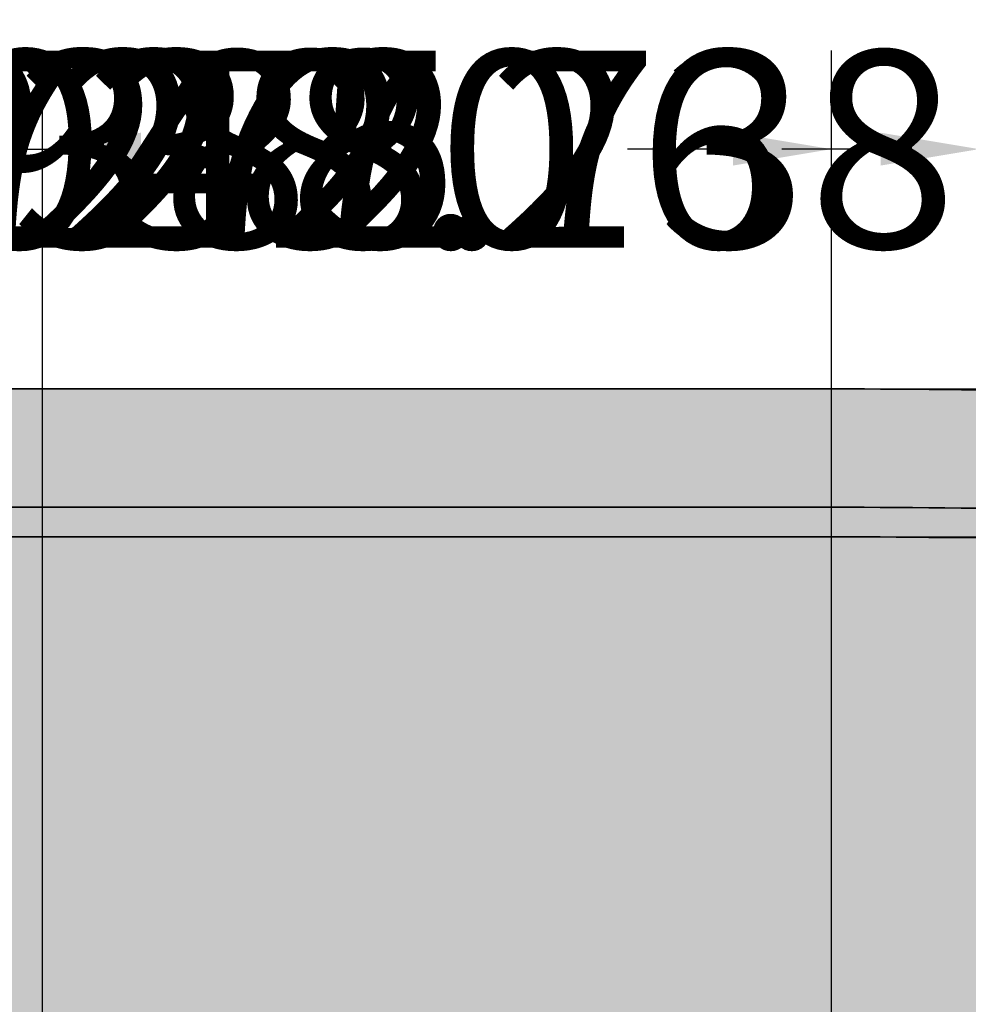
# Model space of a CAD drawing. Units: millimetres. Extents: x 130 to 1021, y 147 to 699.
# Tile 38 of 40: x 550 to 646, y 600 to 699. Entities that reach past the tile are written whole.
import ezdxf

# ---------------------------------------------------------------- set-up
doc = ezdxf.new("R2010")
doc.units = ezdxf.units.MM
doc.header["$MEASUREMENT"] = 0
for name, color, linetype, lineweight in [('A-ANNO-DIMS', 2, 'Continuous', 18), ('A-ELEV', 7, 'Continuous', 35), ('A-ELEV-PATT', 9, 'Continuous', 13)]:
    doc.layers.add(name, color=color, linetype=linetype, lineweight=lineweight)
doc.styles.get("Standard").update_dxf_attribs({"font": 'arial.ttf'})
doc.dimstyles.get("Standard").update_dxf_attribs({"dimtxt": 20, "dimasz": 10, "dimexe": 10, "dimexo": 10, "dimgap": 5, "dimtad": 0, "dimtih": 1, "dimtoh": 1, "dimdec": 0, "dimzin": 0, "dimdsep": 46, "dimtxsty": 'Standard', "dimcen": 5, "dimadec": 0, "dimazin": 0, "dimtfac": 1, "dimtdec": 0, "dimtofl": 0, "dimtmove": 0, "dimatfit": 3, "dimfxl": 1, "dimtolj": 1, "dimtzin": 0, "dimarcsym": 0})

# ---------------------------------------------------------------- blocks, each defined once
blk = doc.blocks.new('*D11')
at = {"layer": 'A-ANNO-DIMS', "color": 0, "lineweight": -2, "transparency": 16777216}
for p, q in [((737.374, 648.699), (737.374, 149.739)), ((299.374, 566.947), (299.374, 149.739)), ((309.374, 159.739), (490.857, 159.739)), ((727.374, 159.739), (545.891, 159.739))]:
    blk.add_line(p, q, dxfattribs=at)
at = {"layer": 'A-ANNO-DIMS', "color": 0, "transparency": 16777216}
for points in [[(309.374, 161.406), (309.374, 158.073), (299.374, 159.739)], [(727.374, 161.406), (727.374, 158.073), (737.374, 159.739)]]:
    blk.add_solid(points, dxfattribs=at)
at = {"layer": 'Defpoints', "color": 0, "transparency": 16777216}
for p in [(737.374, 658.699), (299.374, 576.947), (737.374, 159.739)]:
    blk.add_point(p, dxfattribs=at)
at = {"layer": 'A-ANNO-DIMS', "color": 0, "transparency": 16777216, "insert": (518.374, 159.739), "char_height": 20, "attachment_point": 5}
blk.add_mtext('\\A1;438', dxfattribs=at)
blk = doc.blocks.new('*D22')
at = {"layer": 'A-ANNO-DIMS', "color": 0, "lineweight": -2, "transparency": 16777216}
for p, q in [((447.374, 656.947), (447.374, 696.247)), ((466.767, 403.947), (466.767, 696.247)), ((437.374, 686.247), (427.374, 686.247)), ((476.767, 686.247), (486.767, 686.247))]:
    blk.add_line(p, q, dxfattribs=at)
at = {"layer": 'A-ANNO-DIMS', "color": 0, "transparency": 16777216}
for points in [[(437.374, 687.914), (437.374, 684.581), (447.374, 686.247)], [(476.767, 687.914), (476.767, 684.581), (466.767, 686.247)]]:
    blk.add_solid(points, dxfattribs=at)
at = {"layer": 'Defpoints', "color": 0, "transparency": 16777216}
for p in [(466.767, 686.247), (447.374, 646.947), (466.767, 393.947)]:
    blk.add_point(p, dxfattribs=at)
at = {"layer": 'A-ANNO-DIMS', "color": 0, "transparency": 16777216, "insert": (532.34, 686.247), "char_height": 20, "attachment_point": 5}
blk.add_mtext('\\A1;19.393', dxfattribs=at)
blk = doc.blocks.new('*D23')
at = {"layer": 'A-ANNO-DIMS', "color": 0, "lineweight": -2, "transparency": 16777216}
for p, q in [((466.767, 403.947), (466.767, 696.247)), ((475.988, 209.039), (475.988, 696.247)), ((456.767, 686.247), (446.767, 686.247)), ((485.988, 686.247), (495.988, 686.247))]:
    blk.add_line(p, q, dxfattribs=at)
at = {"layer": 'A-ANNO-DIMS', "color": 0, "transparency": 16777216}
for points in [[(456.767, 687.914), (456.767, 684.581), (466.767, 686.247)], [(485.988, 687.914), (485.988, 684.581), (475.988, 686.247)]]:
    blk.add_solid(points, dxfattribs=at)
at = {"layer": 'Defpoints', "color": 0, "transparency": 16777216}
for p in [(475.988, 686.247), (466.767, 393.947), (475.988, 199.039)]:
    blk.add_point(p, dxfattribs=at)
at = {"layer": 'A-ANNO-DIMS', "color": 0, "transparency": 16777216, "insert": (534.631, 686.247), "char_height": 20, "attachment_point": 5}
blk.add_mtext('\\A1;9.222', dxfattribs=at)
blk = doc.blocks.new('*D24')
at = {"layer": 'A-ANNO-DIMS', "color": 0, "lineweight": -2, "transparency": 16777216}
for p, q in [((475.988, 209.039), (475.988, 696.247)), ((487.374, 671.947), (487.374, 696.247)), ((465.988, 686.247), (455.988, 686.247)), ((497.374, 686.247), (507.374, 686.247))]:
    blk.add_line(p, q, dxfattribs=at)
at = {"layer": 'A-ANNO-DIMS', "color": 0, "transparency": 16777216}
for points in [[(465.988, 687.914), (465.988, 684.581), (475.988, 686.247)], [(497.374, 687.914), (497.374, 684.581), (487.374, 686.247)]]:
    blk.add_solid(points, dxfattribs=at)
at = {"layer": 'Defpoints', "color": 0, "transparency": 16777216}
for p in [(487.374, 686.247), (487.374, 661.947), (475.988, 199.039)]:
    blk.add_point(p, dxfattribs=at)
at = {"layer": 'A-ANNO-DIMS', "color": 0, "transparency": 16777216, "insert": (553.022, 686.247), "char_height": 20, "attachment_point": 5}
blk.add_mtext('\\A1;11.385', dxfattribs=at)
blk = doc.blocks.new('*D25')
at = {"layer": 'A-ANNO-DIMS', "color": 0, "lineweight": -2, "transparency": 16777216}
for p, q in [((487.374, 671.947), (487.374, 696.247)), ((494.102, 506.908), (494.102, 696.247)), ((477.374, 686.247), (467.374, 686.247)), ((504.102, 686.247), (514.102, 686.247))]:
    blk.add_line(p, q, dxfattribs=at)
at = {"layer": 'A-ANNO-DIMS', "color": 0, "transparency": 16777216}
for points in [[(477.374, 687.914), (477.374, 684.581), (487.374, 686.247)], [(504.102, 687.914), (504.102, 684.581), (494.102, 686.247)]]:
    blk.add_solid(points, dxfattribs=at)
at = {"layer": 'Defpoints', "color": 0, "transparency": 16777216}
for p in [(494.102, 686.247), (487.374, 661.947), (494.102, 496.908)]:
    blk.add_point(p, dxfattribs=at)
at = {"layer": 'A-ANNO-DIMS', "color": 0, "transparency": 16777216, "insert": (552.922, 686.247), "char_height": 20, "attachment_point": 5}
blk.add_mtext('\\A1;6.728', dxfattribs=at)
blk = doc.blocks.new('*D26')
at = {"layer": 'A-ANNO-DIMS', "color": 0, "lineweight": -2, "transparency": 16777216}
for p, q in [((494.102, 506.908), (494.102, 696.247)), ((502.374, 593.947), (502.374, 696.247)), ((484.102, 686.247), (474.102, 686.247)), ((512.374, 686.247), (522.374, 686.247))]:
    blk.add_line(p, q, dxfattribs=at)
at = {"layer": 'A-ANNO-DIMS', "color": 0, "transparency": 16777216}
for points in [[(484.102, 687.914), (484.102, 684.581), (494.102, 686.247)], [(512.374, 687.914), (512.374, 684.581), (502.374, 686.247)]]:
    blk.add_solid(points, dxfattribs=at)
at = {"layer": 'Defpoints', "color": 0, "transparency": 16777216}
for p in [(502.374, 686.247), (502.374, 583.947), (494.102, 496.908)]:
    blk.add_point(p, dxfattribs=at)
at = {"layer": 'A-ANNO-DIMS', "color": 0, "transparency": 16777216, "insert": (561.03, 686.247), "char_height": 20, "attachment_point": 5}
blk.add_mtext('\\A1;8.272', dxfattribs=at)
blk = doc.blocks.new('*D27')
at = {"layer": 'A-ANNO-DIMS', "color": 0, "lineweight": -2, "transparency": 16777216}
for p, q in [((502.374, 593.947), (502.374, 696.247)), ((544.635, 396.264), (544.635, 696.247)), ((512.374, 686.247), (534.635, 686.247)), ((544.635, 686.247), (554.635, 686.247))]:
    blk.add_line(p, q, dxfattribs=at)
at = {"layer": 'A-ANNO-DIMS', "color": 0, "transparency": 16777216}
for points in [[(512.374, 687.914), (512.374, 684.581), (502.374, 686.247)], [(534.635, 687.914), (534.635, 684.581), (544.635, 686.247)]]:
    blk.add_solid(points, dxfattribs=at)
at = {"layer": 'Defpoints', "color": 0, "transparency": 16777216}
for p in [(544.635, 686.247), (502.374, 583.947), (544.635, 386.264)]:
    blk.add_point(p, dxfattribs=at)
at = {"layer": 'A-ANNO-DIMS', "color": 0, "transparency": 16777216, "insert": (593.776, 686.247), "char_height": 20, "attachment_point": 5}
blk.add_mtext('\\A1;42.26', dxfattribs=at)
blk = doc.blocks.new('*D28')
at = {"layer": 'A-ANNO-DIMS', "color": 0, "lineweight": -2, "transparency": 16777216}
for p, q in [((544.635, 396.264), (544.635, 696.247)), ((552.374, 593.947), (552.374, 696.247)), ((534.635, 686.247), (524.635, 686.247)), ((562.374, 686.247), (572.374, 686.247))]:
    blk.add_line(p, q, dxfattribs=at)
at = {"layer": 'A-ANNO-DIMS', "color": 0, "transparency": 16777216}
for points in [[(534.635, 687.914), (534.635, 684.581), (544.635, 686.247)], [(562.374, 687.914), (562.374, 684.581), (552.374, 686.247)]]:
    blk.add_solid(points, dxfattribs=at)
at = {"layer": 'Defpoints', "color": 0, "transparency": 16777216}
for p in [(552.374, 686.247), (552.374, 583.947), (544.635, 386.264)]:
    blk.add_point(p, dxfattribs=at)
at = {"layer": 'A-ANNO-DIMS', "color": 0, "transparency": 16777216, "insert": (611.057, 686.247), "char_height": 20, "attachment_point": 5}
blk.add_mtext('\\A1;7.738', dxfattribs=at)
blk = doc.blocks.new('*D29')
at = {"layer": 'A-ANNO-DIMS', "color": 0, "lineweight": -2, "transparency": 16777216}
for p, q in [((552.374, 593.947), (552.374, 696.247)), ((632.374, 593.947), (632.374, 696.247)), ((562.374, 686.247), (573.07, 686.247)), ((622.374, 686.247), (611.678, 686.247))]:
    blk.add_line(p, q, dxfattribs=at)
at = {"layer": 'A-ANNO-DIMS', "color": 0, "transparency": 16777216}
for points in [[(562.374, 687.914), (562.374, 684.581), (552.374, 686.247)], [(622.374, 687.914), (622.374, 684.581), (632.374, 686.247)]]:
    blk.add_solid(points, dxfattribs=at)
at = {"layer": 'Defpoints', "color": 0, "transparency": 16777216}
for p in [(632.374, 686.247), (552.374, 583.947), (632.374, 583.947)]:
    blk.add_point(p, dxfattribs=at)
at = {"layer": 'A-ANNO-DIMS', "color": 0, "transparency": 16777216, "insert": (592.374, 686.247), "char_height": 20, "attachment_point": 5}
blk.add_mtext('\\A1;80', dxfattribs=at)
blk = doc.blocks.new('*D30')
at = {"layer": 'A-ANNO-DIMS', "color": 0, "lineweight": -2, "transparency": 16777216}
for p, q in [((632.374, 593.947), (632.374, 696.247)), ((647.339, 584.979), (647.339, 696.247)), ((622.374, 686.247), (612.374, 686.247)), ((657.339, 686.247), (667.339, 686.247))]:
    blk.add_line(p, q, dxfattribs=at)
at = {"layer": 'A-ANNO-DIMS', "color": 0, "transparency": 16777216}
for points in [[(622.374, 687.914), (622.374, 684.581), (632.374, 686.247)], [(657.339, 687.914), (657.339, 684.581), (647.339, 686.247)]]:
    blk.add_solid(points, dxfattribs=at)
at = {"layer": 'Defpoints', "color": 0, "transparency": 16777216}
for p in [(647.339, 686.247), (632.374, 583.947), (647.339, 574.979)]:
    blk.add_point(p, dxfattribs=at)
at = {"layer": 'A-ANNO-DIMS', "color": 0, "transparency": 16777216, "insert": (712.987, 686.247), "char_height": 20, "attachment_point": 5}
blk.add_mtext('\\A1;14.965', dxfattribs=at)
blk = doc.blocks.new('*D31')
at = {"layer": 'A-ANNO-DIMS', "color": 0, "lineweight": -2, "transparency": 16777216}
for p, q in [((647.339, 584.979), (647.339, 696.247)), ((732.374, 653.96), (732.374, 696.247)), ((637.339, 686.247), (627.339, 686.247)), ((742.374, 686.247), (752.374, 686.247))]:
    blk.add_line(p, q, dxfattribs=at)
at = {"layer": 'A-ANNO-DIMS', "color": 0, "transparency": 16777216}
for points in [[(637.339, 687.914), (637.339, 684.581), (647.339, 686.247)], [(742.374, 687.914), (742.374, 684.581), (732.374, 686.247)]]:
    blk.add_solid(points, dxfattribs=at)
at = {"layer": 'Defpoints', "color": 0, "transparency": 16777216}
for p in [(732.374, 686.247), (732.374, 643.96), (647.339, 574.979)]:
    blk.add_point(p, dxfattribs=at)
at = {"layer": 'A-ANNO-DIMS', "color": 0, "transparency": 16777216, "insert": (689.857, 686.247), "char_height": 20, "attachment_point": 5}
blk.add_mtext('\\A1;85.03', dxfattribs=at)
blk = doc.blocks.new('*D57')
at = {"layer": 'A-ANNO-DIMS', "color": 0, "lineweight": -2, "transparency": 16777216}
for p, q in [((761.674, 606.947), (761.674, 616.947)), ((761.674, 616.947), (771.674, 616.947)), ((497.374, 596.947), (771.674, 596.947)), ((562.374, 583.947), (771.674, 583.947)), ((761.674, 573.947), (761.674, 563.947))]:
    blk.add_line(p, q, dxfattribs=at)
at = {"layer": 'A-ANNO-DIMS', "color": 0, "transparency": 16777216}
for points in [[(760.007, 606.947), (763.34, 606.947), (761.674, 596.947)], [(760.007, 573.947), (763.34, 573.947), (761.674, 583.947)]]:
    blk.add_solid(points, dxfattribs=at)
at = {"layer": 'Defpoints', "color": 0, "transparency": 16777216}
for p in [(487.374, 596.947), (761.674, 596.947), (552.374, 583.947)]:
    blk.add_point(p, dxfattribs=at)
at = {"layer": 'A-ANNO-DIMS', "color": 0, "transparency": 16777216, "insert": (790.057, 616.947), "char_height": 20, "attachment_point": 5}
blk.add_mtext('\\A1;13', dxfattribs=at)
blk = doc.blocks.new('*D58')
at = {"layer": 'A-ANNO-DIMS', "color": 0, "lineweight": -2, "transparency": 16777216}
for p, q in [((761.674, 656.947), (761.674, 666.947)), ((497.374, 646.947), (771.674, 646.947)), ((497.374, 596.947), (771.674, 596.947)), ((761.674, 586.947), (761.674, 576.947))]:
    blk.add_line(p, q, dxfattribs=at)
at = {"layer": 'A-ANNO-DIMS', "color": 0, "transparency": 16777216}
for points in [[(760.007, 656.947), (763.34, 656.947), (761.674, 646.947)], [(760.007, 586.947), (763.34, 586.947), (761.674, 596.947)]]:
    blk.add_solid(points, dxfattribs=at)
at = {"layer": 'Defpoints', "color": 0, "transparency": 16777216}
for p in [(487.374, 646.947), (761.674, 646.947), (487.374, 596.947)]:
    blk.add_point(p, dxfattribs=at)
at = {"layer": 'A-ANNO-DIMS', "color": 0, "transparency": 16777216, "insert": (761.674, 621.947), "char_height": 20, "attachment_point": 5}
blk.add_mtext('\\A1;50', dxfattribs=at)
blk = doc.blocks.new('*D59')
at = {"layer": 'A-ANNO-DIMS', "color": 0, "lineweight": -2, "transparency": 16777216}
for p, q in [((761.674, 671.947), (761.674, 681.947)), ((761.674, 681.947), (771.674, 681.947)), ((497.374, 661.947), (771.674, 661.947)), ((497.374, 646.947), (771.674, 646.947)), ((761.674, 636.947), (761.674, 626.947))]:
    blk.add_line(p, q, dxfattribs=at)
at = {"layer": 'A-ANNO-DIMS', "color": 0, "transparency": 16777216}
for points in [[(760.007, 671.947), (763.34, 671.947), (761.674, 661.947)], [(760.007, 636.947), (763.34, 636.947), (761.674, 646.947)]]:
    blk.add_solid(points, dxfattribs=at)
at = {"layer": 'Defpoints', "color": 0, "transparency": 16777216}
for p in [(487.374, 661.947), (761.674, 661.947), (487.374, 646.947)]:
    blk.add_point(p, dxfattribs=at)
at = {"layer": 'A-ANNO-DIMS', "color": 0, "transparency": 16777216, "insert": (790.132, 681.947), "char_height": 20, "attachment_point": 5}
blk.add_mtext('\\A1;15', dxfattribs=at)

msp = doc.modelspace()

# ---------------------------------------------------------------- hatches: boundary and pattern name
at = {"layer": 'A-ELEV-PATT'}
h = msp.add_hatch(color=256, dxfattribs=at)
h.dxf.hatch_style = 1
h.paths.add_polyline_path([(737.3738, 658.6988, 0.0135961), (632.4019, 661.9473), (607.3738, 661.9473), (487.3738, 661.9473), (487.3738, 649.9473), (607.3738, 649.9473), (632.3794, 649.9473, -0.0136841), (737.3738, 646.6784)])
h.paths.add_polyline_path([(732.3738, 643.9599, 0.0130529), (632.3738, 646.9473), (607.3738, 646.9473), (487.3738, 646.9473), (487.3738, 596.9473), (632.3738, 596.9473, -0.0130529), (732.3738, 593.9599)])
h.paths.add_polyline_path([(737.3738, 593.6732, 0.0137063), (632.3738, 596.9473), (487.3738, 596.9473), (487.3738, 586.9473), (632.355, 586.9473, -0.0137808), (737.3738, 583.6559)])
h.paths.add_polyline_path([(447.3738, 646.9473), (307.3738, 646.9473), (302.3738, 646.9473), (302.3738, 634.9473), (447.3738, 634.9473)])
h.paths.add_polyline_path([(447.3738, 631.9473), (307.3738, 631.9473), (307.3738, 586.9473), (447.3738, 586.9473)])
h.paths.add_polyline_path([(447.3738, 586.9473), (307.3738, 586.9473), (302.3738, 586.9473), (302.3738, 576.9473), (447.3738, 576.9473)])
h.paths.add_polyline_path([(447.3738, 573.9473), (367.3738, 573.9473), (367.3738, 539.9473), (447.3738, 539.9473)])
h.paths.add_polyline_path([(447.3738, 537.9473), (367.3738, 537.9473), (367.3738, 507.9473), (400.392, 507.4253, -0.001728), (401.3281, 507.6451, -0.5220025), (425.6117, 511.0391, -0.0391849), (447.3738, 510.4359), (447.3738, 510.7883)])
h.paths.add_polyline_path([(394.7238, 505.9473), (367.3738, 505.9473), (367.3738, 476.9473, -0.0146512), (375.8501, 480.2159), (376.1506, 499.2266, -0.0355419)])
h.paths.add_polyline_path([(632.3738, 583.9473), (552.3738, 583.9473), (552.3738, 550.9473), (632.3738, 550.9473)])
h.paths.add_polyline_path([(632.3738, 548.9473), (552.3738, 548.9473), (552.3738, 515.9473), (632.3738, 515.9473)])
h.paths.add_polyline_path([(632.3738, 513.9473), (552.3738, 513.9473), (552.3738, 476.9473), (632.3738, 476.9473)])
h.paths.add_polyline_path([(737.3738, 473.6903, 0.0136326), (632.3926, 476.9473), (552.3738, 476.9473), (487.3738, 476.9473), (487.3738, 466.9473), (632.3738, 466.9473, -0.0137063), (737.3738, 463.6732)])
h.paths.add_polyline_path([(732.3738, 460.9552, 0.0130741), (632.3681, 463.9473), (487.3738, 463.9473), (487.3738, 407.735, -0.0032286), (489.3544, 406.9473), (632.3926, 406.9473, -0.0129826), (732.3738, 403.9755)])
h.paths.add_polyline_path([(487.3738, 463.9473, 0.20133), (367.3738, 463.9473), (367.3738, 407.735, -0.1882031), (487.3738, 407.735)])
h.paths.add_polyline_path([(367.3738, 476.9473), (367.3738, 466.9473, -0.2013309), (487.3738, 466.9473), (487.3738, 476.9473, 0.20133)])
h.paths.add_polyline_path([(367.3738, 463.9473), (307.3738, 463.9473), (307.3738, 401.9473), (357.9413, 401.9473), (367.3738, 407.735)])
h.paths.add_polyline_path([(367.3738, 476.9473), (302.3738, 476.9473), (302.3738, 466.9473), (367.3738, 466.9473)])
h.paths.add_polyline_path([(632.8184, 366.9453), (552.3738, 366.9453), (552.3738, 393.9473), (632.8184, 393.9473)])
h.paths.add_polyline_path([(632.8184, 357.2114), (632.8184, 363.9453), (552.3738, 363.9453), (552.3738, 357.2114), (552.3738, 336.9453), (632.8184, 336.9453)])
h.paths.add_polyline_path([(632.8184, 333.9453), (552.3738, 333.9453), (552.3738, 306.9453), (632.8184, 306.9453)])
h.paths.add_polyline_path([(632.8184, 303.9453), (552.3738, 303.9453), (552.3738, 273.9473), (632.355, 273.9473, 0.0000608), (632.8184, 273.9491)])
h.paths.add_polyline_path([(737.3738, 403.6903, 0.0136326), (632.3926, 406.9473), (489.3544, 406.9473, 0.1915481), (367.3738, 407.735), (367.3738, 396.9473, -0.2013309), (487.3738, 396.9473), (632.3738, 396.9473, -0.0137063), (737.3738, 393.6732)])
h.paths.add_polyline_path([(357.9413, 401.9473), (307.3738, 401.9473), (307.3738, 391.9473), (357.9413, 391.9473)])
h.paths.add_polyline_path([(357.9413, 357.2114), (357.9413, 388.9473), (307.3738, 388.9473), (307.3738, 357.2114), (307.3738, 273.9473), (357.9413, 273.9473)])
h.paths.add_polyline_path([(732.3738, 263.93, -0.0130317), (632.3794, 260.9473), (466.7667, 260.9473), (466.7667, 240.9473), (469.8406, 236.978), (469.8406, 221.978), (472.9145, 218.0087), (472.9145, 213.9473), (607.3738, 213.9473), (732.3738, 213.9473)])
h.paths.add_polyline_path([(732.3738, 290.889), (722.479, 290.889), (722.479, 301.889), (732.3738, 301.889), (732.3738, 305.889), (722.479, 305.889), (722.479, 316.889), (732.3738, 316.889), (732.3738, 320.889), (722.479, 320.889), (722.479, 331.889), (732.3738, 331.889), (732.3738, 335.889), (722.479, 335.889), (722.479, 346.889), (732.3738, 346.889), (732.3738, 350.889), (722.479, 350.889), (722.479, 361.889), (732.3738, 361.889), (732.3738, 365.889), (722.479, 365.889), (722.479, 376.889), (732.3738, 376.889), (732.3738, 380.889), (722.479, 380.889), (722.479, 391.4848, 0.0005233), (718.479, 391.6843), (718.479, 380.889), (707.479, 380.889), (707.479, 392.1896, 0.0005231), (703.479, 392.3576), (703.479, 380.889), (692.479, 380.889), (692.479, 392.7765, 0.0005229), (688.479, 392.9131), (688.479, 380.889), (677.479, 380.889), (677.479, 393.2456, 0.0005228), (673.479, 393.3508), (673.479, 380.889), (662.479, 380.889), (662.479, 393.597, 0.0005227), (658.479, 393.6709), (658.479, 380.889), (647.479, 380.889), (647.479, 393.8308, 0.0005226), (643.479, 393.8732), (643.479, 380.889), (632.8184, 380.889), (632.8184, 376.889), (643.479, 376.889), (643.479, 365.889), (632.8184, 365.889), (632.8184, 361.889), (643.479, 361.889), (643.479, 350.889), (632.8184, 350.889), (632.8184, 346.889), (643.479, 346.889), (643.479, 335.889), (632.8184, 335.889), (632.8184, 331.889), (643.479, 331.889), (643.479, 320.889), (632.8184, 320.889), (632.8184, 316.889), (643.479, 316.889), (643.479, 305.889), (632.8184, 305.889), (632.8184, 301.889), (643.479, 301.889), (643.479, 290.889), (632.8184, 290.889), (632.8184, 286.889), (643.479, 286.889), (643.479, 274.0217, 0.0005246), (647.479, 274.0643), (647.479, 286.889), (658.479, 286.889), (658.479, 274.2248, 0.0005246), (662.479, 274.2989), (662.479, 286.889), (673.479, 286.889), (673.479, 274.546, 0.0005247), (677.479, 274.6516), (677.479, 286.889), (688.479, 286.889), (688.479, 274.9853, 0.0005248), (692.479, 275.1224), (692.479, 286.889), (703.479, 286.889), (703.479, 275.5429, 0.000525), (707.479, 275.7115), (707.479, 286.889), (718.479, 286.889), (718.479, 276.2187, 0.0005252), (722.479, 276.4189), (722.479, 286.889), (732.3738, 286.889)])
h.paths.add_polyline_path([(718.479, 290.889), (707.479, 290.889), (707.479, 301.889), (718.479, 301.889)], flags=16)
h.paths.add_polyline_path([(703.479, 290.889), (692.479, 290.889), (692.479, 301.889), (703.479, 301.889)], flags=16)
h.paths.add_polyline_path([(718.479, 305.889), (707.479, 305.889), (707.479, 316.889), (718.479, 316.889)], flags=16)
h.paths.add_polyline_path([(703.479, 305.889), (692.479, 305.889), (692.479, 316.889), (703.479, 316.889)], flags=16)
h.paths.add_polyline_path([(688.479, 290.889), (677.479, 290.889), (677.479, 301.889), (688.479, 301.889)], flags=16)
h.paths.add_polyline_path([(718.479, 320.889), (707.479, 320.889), (707.479, 331.889), (718.479, 331.889)], flags=16)
h.paths.add_polyline_path([(688.479, 305.889), (677.479, 305.889), (677.479, 316.889), (688.479, 316.889)], flags=16)
h.paths.add_polyline_path([(703.479, 320.889), (692.479, 320.889), (692.479, 331.889), (703.479, 331.889)], flags=16)
h.paths.add_polyline_path([(688.479, 320.889), (677.479, 320.889), (677.479, 331.889), (688.479, 331.889)], flags=16)
h.paths.add_polyline_path([(673.479, 290.889), (662.479, 290.889), (662.479, 301.889), (673.479, 301.889)], flags=16)
h.paths.add_polyline_path([(718.479, 335.889), (707.479, 335.889), (707.479, 346.889), (718.479, 346.889)], flags=16)
h.paths.add_polyline_path([(673.479, 305.889), (662.479, 305.889), (662.479, 316.889), (673.479, 316.889)], flags=16)
h.paths.add_polyline_path([(703.479, 335.889), (692.479, 335.889), (692.479, 346.889), (703.479, 346.889)], flags=16)
h.paths.add_polyline_path([(673.479, 320.889), (662.479, 320.889), (662.479, 331.889), (673.479, 331.889)], flags=16)
h.paths.add_polyline_path([(688.479, 335.889), (677.479, 335.889), (677.479, 346.889), (688.479, 346.889)], flags=16)
h.paths.add_polyline_path([(658.479, 290.889), (647.479, 290.889), (647.479, 301.889), (658.479, 301.889)], flags=16)
h.paths.add_polyline_path([(718.479, 350.889), (707.479, 350.889), (707.479, 361.889), (718.479, 361.889)], flags=16)
h.paths.add_polyline_path([(658.479, 305.889), (647.479, 305.889), (647.479, 316.889), (658.479, 316.889)], flags=16)
h.paths.add_polyline_path([(703.479, 350.889), (692.479, 350.889), (692.479, 361.889), (703.479, 361.889)], flags=16)
h.paths.add_polyline_path([(673.479, 335.889), (662.479, 335.889), (662.479, 346.889), (673.479, 346.889)], flags=16)
h.paths.add_polyline_path([(658.479, 320.889), (647.479, 320.889), (647.479, 331.889), (658.479, 331.889)], flags=16)
h.paths.add_polyline_path([(688.479, 350.889), (677.479, 350.889), (677.479, 361.889), (688.479, 361.889)], flags=16)
h.paths.add_polyline_path([(718.479, 365.889), (707.479, 365.889), (707.479, 376.889), (718.479, 376.889)], flags=16)
h.paths.add_polyline_path([(658.479, 335.889), (647.479, 335.889), (647.479, 346.889), (658.479, 346.889)], flags=16)
h.paths.add_polyline_path([(673.479, 350.889), (662.479, 350.889), (662.479, 361.889), (673.479, 361.889)], flags=16)
h.paths.add_polyline_path([(703.479, 365.889), (692.479, 365.889), (692.479, 376.889), (703.479, 376.889)], flags=16)
h.paths.add_polyline_path([(688.479, 365.889), (677.479, 365.889), (677.479, 376.889), (688.479, 376.889)], flags=16)
h.paths.add_polyline_path([(658.479, 350.889), (647.479, 350.889), (647.479, 361.889), (658.479, 361.889)], flags=16)
h.paths.add_polyline_path([(673.479, 365.889), (662.479, 365.889), (662.479, 376.889), (673.479, 376.889)], flags=16)
h.paths.add_polyline_path([(658.479, 365.889), (647.479, 365.889), (647.479, 376.889), (658.479, 376.889)], flags=16)
h.paths.add_polyline_path([(732.3738, 503.9786), (722.3392, 503.9786), (722.3392, 514.9786), (732.3738, 514.9786), (732.3738, 518.9786), (722.3392, 518.9786), (722.3392, 529.9786), (732.3738, 529.9786), (732.3738, 533.9786), (722.3392, 533.9786), (722.3392, 544.9786), (732.3738, 544.9786), (732.3738, 546.9473), (732.3738, 548.9786), (722.3392, 548.9786), (722.3392, 559.9786), (732.3738, 559.9786), (732.3738, 563.9786), (722.3392, 563.9786), (722.3392, 574.9786), (732.3738, 574.9786), (732.3738, 578.9786), (722.3392, 578.9786), (722.3392, 581.4789, 0.000526), (718.3392, 581.6791), (718.3392, 578.9786), (707.3392, 578.9786), (707.3392, 582.1863, 0.0005258), (703.3392, 582.355), (703.3392, 578.9786), (692.3392, 578.9786), (692.3392, 582.7752, 0.0005257), (688.3392, 582.9123), (688.3392, 578.9786), (677.3392, 578.9786), (677.3392, 583.2457, 0.0005255), (673.3392, 583.3512), (673.3392, 578.9786), (662.3392, 578.9786), (662.3392, 583.5978, 0.0005254), (658.3392, 583.6718), (658.3392, 578.9786), (647.3392, 578.9786), (647.3392, 583.8317, 0.0005254), (643.3392, 583.8741), (643.3392, 578.9786), (632.3738, 578.9786), (632.3738, 574.9786), (643.3392, 574.9786), (643.3392, 563.9786), (632.3738, 563.9786), (632.3738, 559.9786), (643.3392, 559.9786), (643.3392, 548.9786), (632.3738, 548.9786), (632.3738, 544.9786), (643.3392, 544.9786), (643.3392, 533.9786), (632.3738, 533.9786), (632.3738, 529.9786), (643.3392, 529.9786), (643.3392, 518.9786), (632.3738, 518.9786), (632.3738, 515.9473), (632.3738, 514.9786), (643.3392, 514.9786), (643.3392, 503.9786), (632.3738, 503.9786), (632.3738, 499.9786), (643.3392, 499.9786), (643.3392, 488.9786), (632.3738, 488.9786), (632.3738, 484.9786), (643.3392, 484.9786), (643.3392, 476.8751, -0.0005191), (647.3392, 476.8332), (647.3392, 484.9786), (658.3392, 484.9786), (658.3392, 476.6752, -0.0005192), (662.3392, 476.6022), (662.3392, 484.9786), (673.3392, 484.9786), (673.3392, 476.3585, -0.0005193), (677.3392, 476.2543), (677.3392, 484.9786), (688.3392, 484.9786), (688.3392, 475.9248, -0.0005194), (692.3392, 475.7894), (692.3392, 484.9786), (703.3392, 484.9786), (703.3392, 475.3741, -0.0005195), (707.3392, 475.2075), (707.3392, 484.9786), (718.3392, 484.9786), (718.3392, 474.7064, -0.0005197), (722.3392, 474.5086), (722.3392, 484.9786), (732.3738, 484.9786), (732.3738, 488.9786), (722.3392, 488.9786), (722.3392, 499.9786), (732.3738, 499.9786)])
h.paths.add_polyline_path([(718.3392, 503.9786), (707.3392, 503.9786), (707.3392, 514.9786), (718.3392, 514.9786)], flags=16)
h.paths.add_polyline_path([(718.3392, 499.9786), (718.3392, 488.9786), (707.3392, 488.9786), (707.3392, 499.9786)], flags=16)
h.paths.add_polyline_path([(718.3392, 518.9786), (707.3392, 518.9786), (707.3392, 529.9786), (718.3392, 529.9786)], flags=16)
h.paths.add_polyline_path([(703.3392, 503.9786), (692.3392, 503.9786), (692.3392, 514.9786), (703.3392, 514.9786)], flags=16)
h.paths.add_polyline_path([(703.3392, 499.9786), (703.3392, 488.9786), (692.3392, 488.9786), (692.3392, 499.9786)], flags=16)
h.paths.add_polyline_path([(703.3392, 518.9786), (692.3392, 518.9786), (692.3392, 529.9786), (703.3392, 529.9786)], flags=16)
h.paths.add_polyline_path([(718.3392, 533.9786), (707.3392, 533.9786), (707.3392, 544.9786), (718.3392, 544.9786)], flags=16)
h.paths.add_polyline_path([(688.3392, 503.9786), (677.3392, 503.9786), (677.3392, 514.9786), (688.3392, 514.9786)], flags=16)
h.paths.add_polyline_path([(688.3392, 499.9786), (688.3392, 488.9786), (677.3392, 488.9786), (677.3392, 499.9786)], flags=16)
h.paths.add_polyline_path([(703.3392, 533.9786), (692.3392, 533.9786), (692.3392, 544.9786), (703.3392, 544.9786)], flags=16)
h.paths.add_polyline_path([(688.3392, 518.9786), (677.3392, 518.9786), (677.3392, 529.9786), (688.3392, 529.9786)], flags=16)
h.paths.add_polyline_path([(688.3392, 533.9786), (677.3392, 533.9786), (677.3392, 544.9786), (688.3392, 544.9786)], flags=16)
h.paths.add_polyline_path([(718.3392, 548.9786), (707.3392, 548.9786), (707.3392, 559.9786), (718.3392, 559.9786)], flags=16)
h.paths.add_polyline_path([(673.3392, 503.9786), (662.3392, 503.9786), (662.3392, 514.9786), (673.3392, 514.9786)], flags=16)
h.paths.add_polyline_path([(673.3392, 499.9786), (673.3392, 488.9786), (662.3392, 488.9786), (662.3392, 499.9786)], flags=16)
h.paths.add_polyline_path([(703.3392, 548.9786), (692.3392, 548.9786), (692.3392, 559.9786), (703.3392, 559.9786)], flags=16)
h.paths.add_polyline_path([(673.3392, 518.9786), (662.3392, 518.9786), (662.3392, 529.9786), (673.3392, 529.9786)], flags=16)
h.paths.add_polyline_path([(688.3392, 548.9786), (677.3392, 548.9786), (677.3392, 559.9786), (688.3392, 559.9786)], flags=16)
h.paths.add_polyline_path([(673.3392, 533.9786), (662.3392, 533.9786), (662.3392, 544.9786), (673.3392, 544.9786)], flags=16)
h.paths.add_polyline_path([(718.3392, 563.9786), (707.3392, 563.9786), (707.3392, 574.9786), (718.3392, 574.9786)], flags=16)
h.paths.add_polyline_path([(658.3392, 503.9786), (647.3392, 503.9786), (647.3392, 514.9786), (658.3392, 514.9786)], flags=16)
h.paths.add_polyline_path([(658.3392, 499.9786), (658.3392, 488.9786), (647.3392, 488.9786), (647.3392, 499.9786)], flags=16)
h.paths.add_polyline_path([(703.3392, 563.9786), (692.3392, 563.9786), (692.3392, 574.9786), (703.3392, 574.9786)], flags=16)
h.paths.add_polyline_path([(658.3392, 518.9786), (647.3392, 518.9786), (647.3392, 529.9786), (658.3392, 529.9786)], flags=16)
h.paths.add_polyline_path([(673.3392, 548.9786), (662.3392, 548.9786), (662.3392, 559.9786), (673.3392, 559.9786)], flags=16)
h.paths.add_polyline_path([(688.3392, 563.9786), (677.3392, 563.9786), (677.3392, 574.9786), (688.3392, 574.9786)], flags=16)
h.paths.add_polyline_path([(658.3392, 533.9786), (647.3392, 533.9786), (647.3392, 544.9786), (658.3392, 544.9786)], flags=16)
h.paths.add_polyline_path([(673.3392, 563.9786), (662.3392, 563.9786), (662.3392, 574.9786), (673.3392, 574.9786)], flags=16)
h.paths.add_polyline_path([(658.3392, 548.9786), (647.3392, 548.9786), (647.3392, 559.9786), (658.3392, 559.9786)], flags=16)
h.paths.add_polyline_path([(658.3392, 563.9786), (647.3392, 563.9786), (647.3392, 574.9786), (658.3392, 574.9786)], flags=16)
h = msp.add_hatch(color=256, dxfattribs=at)
h.dxf.hatch_style = 1
h.paths.add_polyline_path([(447.3738, 634.9473), (302.3738, 634.9473), (302.3738, 631.9473), (307.3738, 631.9473), (447.3738, 631.9473)])
h.paths.add_polyline_path([(487.3738, 646.9473), (487.3738, 649.9473), (447.3738, 634.9473), (447.3738, 631.9473)])
h.paths.add_polyline_path([(632.3794, 649.9473), (607.3738, 649.9473), (487.3738, 649.9473), (487.3738, 646.9473), (607.3738, 646.9473), (632.3738, 646.9473, -0.0137063), (737.3738, 643.6732), (737.3738, 646.6784, 0.0136841)])

# ---------------------------------------------------------------- linework, layer by layer
at = {"layer": 'A-ELEV'}
for p, q in [((607.3738, 661.9473), (487.3738, 661.9473)), ((607.3738, 661.9473), (632.3738, 661.9473)), ((607.3738, 649.9473), (487.3738, 649.9473)), ((607.3738, 649.9473), (632.3738, 649.9473)), ((607.3738, 646.9473), (487.3738, 646.9473)), ((607.3738, 646.9473), (632.3738, 646.9473))]:
    msp.add_line(p, q, dxfattribs=at)
for radius, start in [(1931.4697, 86.6695688), (1919.4697, 86.6487242), (1916.4697, 86.6434721)]:
    msp.add_arc((625.1665, -1269.5089), radius, start, 89.784526, dxfattribs=at)

# ---------------------------------------------------------------- dimensions: what is measured, and where the dimension line sits
at = {"layer": 'A-ANNO-DIMS'}
for base, p1, p2, override, picture, middle in [((466.7667, 686.2473), (447.3738, 646.9473), (466.7667, 393.9473), {"dimdec": 3, "dimlfac": 1, "dimrnd": 0, "dimzin": 0, "dimdsep": 46, "dimlunit": 2}, '*D22', (532.3397, 686.2473)), ((475.9885, 686.2473), (466.7667, 393.9473), (475.9885, 199.0395), {"dimdec": 3, "dimlfac": 1, "dimrnd": 0, "dimzin": 0, "dimdsep": 46, "dimlunit": 2}, '*D23', (534.631, 686.2473)), ((487.3738, 686.2473), (475.9885, 199.0395), (487.3738, 661.9473), {"dimdec": 3, "dimlfac": 1, "dimrnd": 0, "dimzin": 0, "dimdsep": 46, "dimlunit": 2}, '*D24', (553.0218, 686.2473)), ((494.10227, 686.2473), (487.37378, 661.9473), (494.10227, 496.90803), {"dimdec": 3, "dimlfac": 1, "dimrnd": 0, "dimzin": 0, "dimdsep": 46, "dimlunit": 2}, '*D25', (552.92219, 686.2473)), ((502.37378, 686.2473), (494.10227, 496.90803), (502.37378, 583.9473), {"dimdec": 3, "dimlfac": 1, "dimrnd": 0, "dimzin": 0, "dimdsep": 46, "dimlunit": 2}, '*D26', (561.02999, 686.2473)), ((544.6354, 686.2473), (502.3738, 583.9473), (544.6354, 386.2639), {"dimdec": 2, "dimlfac": 1, "dimrnd": 0, "dimzin": 0, "dimdsep": 46, "dimlunit": 2}, '*D27', (593.776, 686.2473)), ((552.3738, 686.2473), (544.6354, 386.2639), (552.3738, 583.9473), {"dimdec": 3, "dimlfac": 1, "dimrnd": 0, "dimzin": 0, "dimdsep": 46, "dimlunit": 2}, '*D28', (611.0573, 686.2473)), ((632.3738, 686.2473), (552.3738, 583.9473), (632.3738, 583.9473), {"dimdec": 0, "dimlfac": 1, "dimrnd": 0, "dimzin": 0, "dimdsep": 46, "dimlunit": 2}, '*D29', (592.3738, 686.2473)), ((647.3392, 686.2473), (632.3738, 583.9473), (647.3392, 574.9786), {"dimdec": 3, "dimlfac": 1, "dimrnd": 0, "dimzin": 0, "dimdsep": 46, "dimlunit": 2}, '*D30', (712.9873, 686.2473)), ((732.3738, 686.2473), (647.3392, 574.9786), (732.3738, 643.9599), {"dimdec": 2, "dimlfac": 1, "dimrnd": 0, "dimzin": 0, "dimdsep": 46, "dimlunit": 2}, '*D31', (689.8565, 686.2473)), ((737.3738, 159.7395), (299.3738, 576.9473), (737.3738, 658.6988), {"dimdec": 0, "dimlfac": 1, "dimrnd": 0, "dimzin": 0, "dimdsep": 46, "dimlunit": 2}, '*D11', (518.3738, 159.7395))]:
    dim = msp.add_linear_dim(base=base, p1=p1, p2=p2, dimstyle='Standard', override=override, dxfattribs=at)
    dim.commit()
    dim.dimension.update_dxf_attribs({"geometry": picture, "text_midpoint": middle})
for base, p1, p2, picture, middle in [((761.6738, 661.9473), (487.3738, 646.9473), (487.3738, 661.9473), '*D59', (790.1322, 681.9473)), ((761.6738, 646.9473), (487.3738, 596.9473), (487.3738, 646.9473), '*D58', (761.6738, 621.9473)), ((761.6738, 596.9473), (552.3738, 583.9473), (487.3738, 596.9473), '*D57', (790.0571, 616.9473))]:
    dim = msp.add_linear_dim(base=base, p1=p1, p2=p2, angle=90, dimstyle='Standard', override={"dimdec": 0, "dimlfac": 1, "dimrnd": 0, "dimzin": 0, "dimdsep": 46, "dimlunit": 2}, dxfattribs=at)
    dim.commit()
    dim.dimension.update_dxf_attribs({"geometry": picture, "text_midpoint": middle})

doc.saveas('drawing.dxf')
